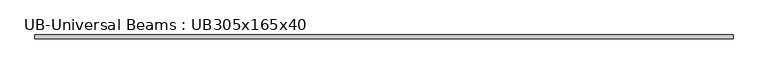
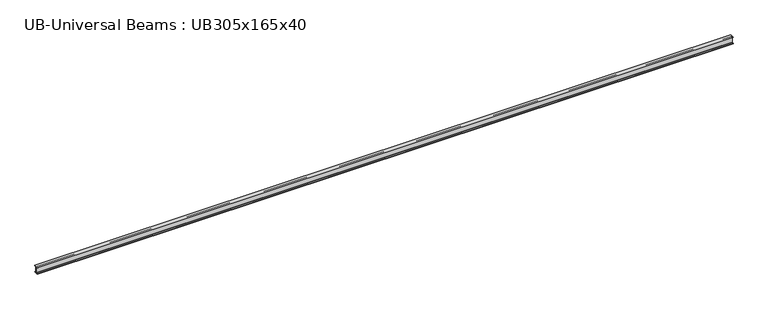
"""IFC4 building model written with IfcOpenShell, lengths in millimetres: beam geometry, UB-Universal Beams : UB305x165x40."""

from ifc_helpers import new_model, si_unit, point, frame, frame_2d, origin, place, context, project, spatial, polyline, circle_curve, trimmed, segment, composite_curve, outline, extrude, source, transform, mapped, element, save


def ub_universal_beams_ub305x165x40_0aabe8ba(model_context):
    return source(origin(), model_context, "Body", "SweptSolid", [
        extrude(outline(composite_curve([segment(polyline([(82.5, -141.5), (82.5, -151.7), (-82.5, -151.7), (-82.5, -141.5), (-11.9, -141.5)]), True, "CONTINUOUS"), segment(trimmed(circle_curve(frame_2d((-11.9, -132.6)), 8.9), [point((-11.9, -141.5))], [point((-3.0, -132.6))], True, "CARTESIAN"), True, "CONTINUOUS"), segment(polyline([(-3.0, -132.6), (-3.0, 132.6)]), True, "CONTINUOUS"), segment(trimmed(circle_curve(frame_2d((-11.9, 132.6)), 8.9), [point((-3.0, 132.6))], [point((-11.9, 141.5))], True, "CARTESIAN"), True, "CONTINUOUS"), segment(polyline([(-11.9, 141.5), (-82.5, 141.5), (-82.5, 151.7), (82.5, 151.7), (82.5, 141.5), (11.9, 141.5)]), True, "CONTINUOUS"), segment(trimmed(circle_curve(frame_2d((11.9, 132.6)), 8.9), [point((11.9, 141.5))], [point((3.0, 132.6))], True, "CARTESIAN"), True, "CONTINUOUS"), segment(polyline([(3.0, 132.6), (3.0, -132.6)]), True, "CONTINUOUS"), segment(trimmed(circle_curve(frame_2d((11.9, -132.6)), 8.9), [point((3.0, -132.6))], [point((11.9, -141.5))], True, "CARTESIAN"), True, "CONTINUOUS"), segment(polyline([(11.9, -141.5), (82.5, -141.5)]), True, "CONTINUOUS")], self_intersect=False)), frame((-15322.5, 0.0, 0.0), z_axis=(1.0, 0.0, 0.0), x_axis=(0.0, 1.0, 0.0)), (0.0, 0.0, 1.0), 30645.0),
    ])


if __name__ == "__main__":
    model = new_model("IFC4")
    model_context = context("Model", 3, world=origin())
    ifc_project = project(units=[si_unit("LENGTHUNIT", "METRE", prefix="MILLI")], contexts=[model_context])
    site = spatial("IfcSite", under=ifc_project)
    building = spatial("IfcBuilding", under=site)
    placement = place(None, origin())
    ub_universal_beams_ub305x165x40_shape = ub_universal_beams_ub305x165x40_0aabe8ba(model_context)
    element("IfcBeam", 1, ObjectType="UB-Universal Beams : UB305x165x40", at=placement, inside=building, context=model_context, shape_type="MappedRepresentation", body=[
        mapped(ub_universal_beams_ub305x165x40_shape, transform((0.0, 0.0, 0.0), x_axis=(1.0, 0.0, 0.0), y_axis=(0.0, 1.0, 0.0), z_axis=(0.0, 0.0, 1.0))),
    ])
    save(model, "model.ifc")

# Revit data of these elements
# Type "UB-Universal Beams : UB305x165x40"
#   Section Name Key = "UB305X165X40"
#   Width = 16.5 cm
#   Web Thickness = 0.6 cm
#   Web Fillet = 0.89 cm
#   Warping Constant = 164000.0 cm⁶
#   Torsional Moment of Inertia = 14.70 cm⁴
#   Section Area = 51.3 cm²
#   Plastic Modulus weak axis = 142.0 cm³
#   Plastic Modulus strong axis = 623.0 cm³
#   Nominal Weight = 40.2999 kgf/m
#   Moment of Inertia weak axis = 764.00 cm⁴
#   Moment of Inertia strong axis = 8503.00 cm⁴
#   Height = 30.34 cm
#   Flange Thickness = 1.02 cm
#   Elastic Modulus weak axis = 92.6 cm³
#   Elastic Modulus strong axis = 560.0 cm³
#   Centroid Vertical = 15.17 cm
#   Centroid Horizontal = 8.25 cm
#   Bolt Spacing = 9.0 cm
#   Length [instance default] = 1500 mm
#   Structural Material [instance default] = Metal - Steel 43-275
#   Type Comments = ""
#   Assembly Code = ""
# Element 1 (IfcBeam, "UB-Universal Beams : UB305x165x40")
#   Materials on its faces: "Metal - Steel 43-275"
# Materials
#   "Metal - Steel 43-275": class "Metal", colour RGB 247 247 247, transparency 0, Cost = 0
